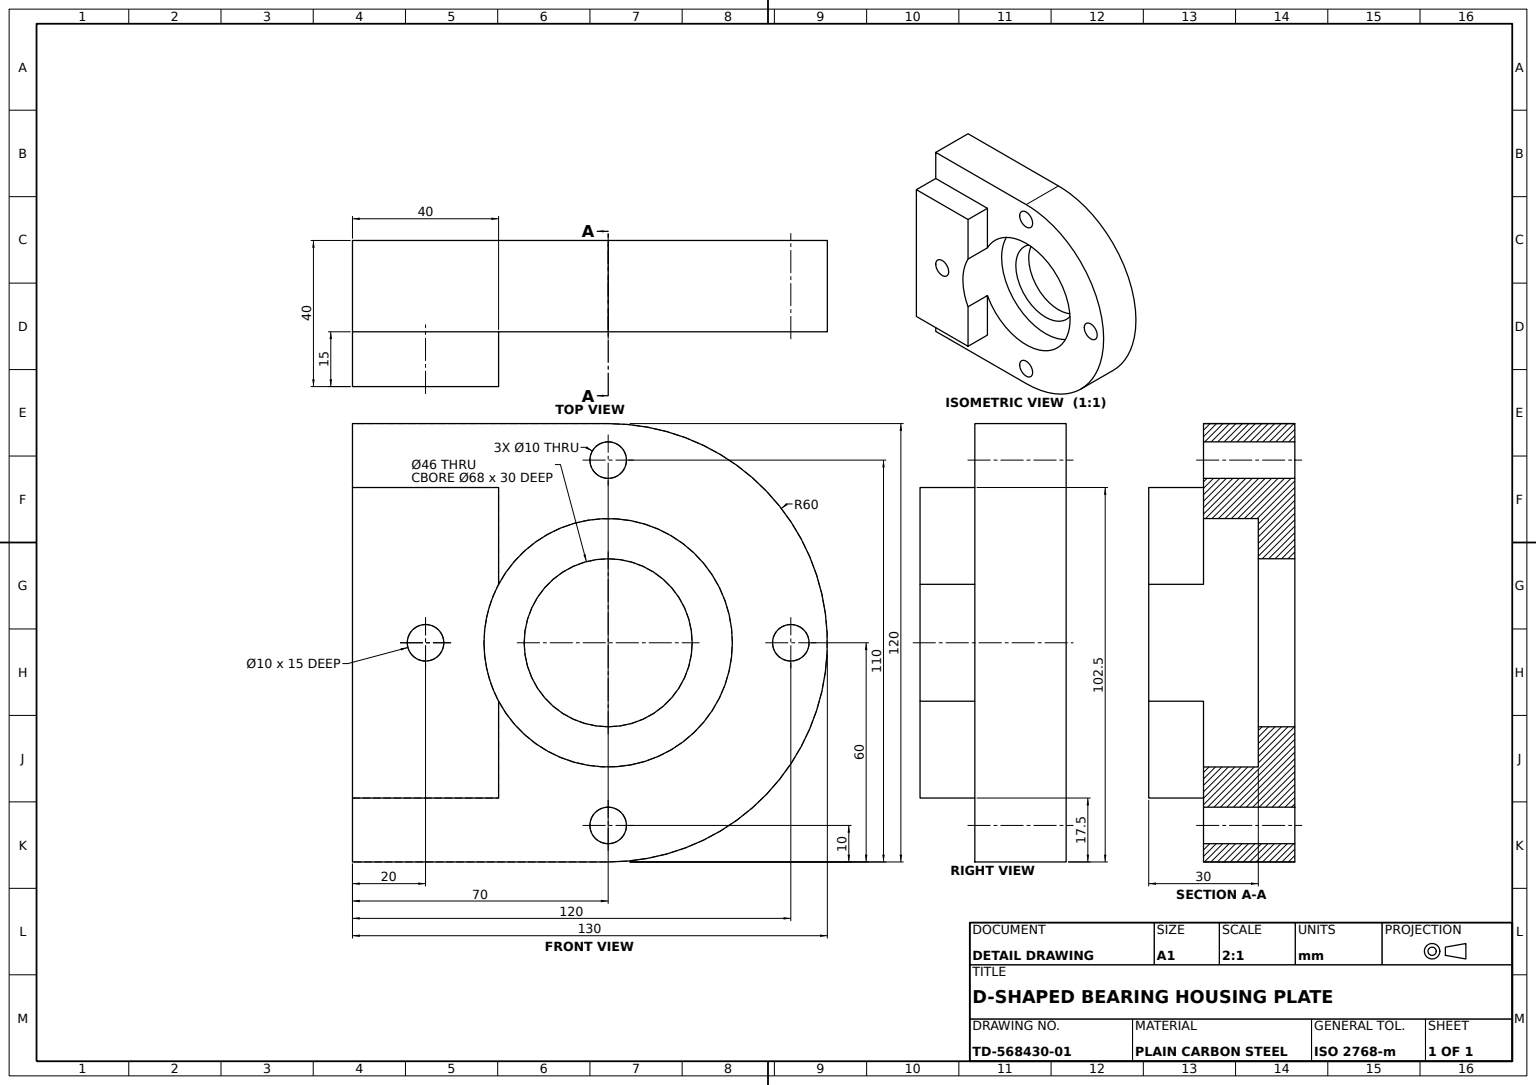
from build123d import *
from build123d.topology import SkipClean

# Parameters (mm, degrees)
BASE_PLATE_DEPTH           = 25
SIDE_BLOCK_SKETCH_W        = 40
SIDE_BLOCK_SKETCH_H        = 85
SIDE_BLOCK_DEPTH           = 15
COUNTERBORE_68_SKETCH_R    = 34
COUNTERBORE_68_DEPTH       = 15
BLOCK_RELIEF_68_DEPTH      = 15
BORE_46_SKETCH_R           = 23
BORE_46_DEPTH              = 15
BLOCK_HOLE_10_SKETCH_R     = 5
BLOCK_HOLE_10_DEPTH        = 15
MOUNTING_HOLES_SKETCH_R    = 5
MOUNTING_HOLES_3X_10_DEPTH = 25


with BuildPart() as part:
    # Base Plate Sketch → Base Plate (new body)
    with BuildSketch(Plane.XY):
        with BuildLine():
            Line((0, 0), (70, 0))
            ThreePointArc((70, 0), (130, 60), (70, 120))
            Line((70, 120), (0, 120))
            Line((0, 120), (0, 0))
        make_face()
    extrude(amount=BASE_PLATE_DEPTH)

    # Side Block Sketch → Side Block (add)
    with BuildSketch(Plane.XY.offset(25)):
        with Locations((20, 60)):
            Rectangle(SIDE_BLOCK_SKETCH_W, SIDE_BLOCK_SKETCH_H)
    extrude(amount=SIDE_BLOCK_DEPTH)

    # Counterbore Ø68 Sketch → Counterbore Ø68 (cut)
    with BuildSketch(Plane.XY.offset(25)):
        with Locations((70, 60)):
            Circle(COUNTERBORE_68_SKETCH_R)
    extrude(amount=-COUNTERBORE_68_DEPTH, mode=Mode.SUBTRACT)

    # Block Relief Ø68 Sketch → Block Relief Ø68 (cut)
    with SkipClean():  # the faces are left unmerged after this step: merging them gives an invalid solid
        with BuildSketch(Plane.XY.offset(40)):
            with BuildLine():
                Line((40, 76), (40, 44))
                ThreePointArc((40, 44), (36, 60), (40, 76))
            make_face()
        extrude(amount=-BLOCK_RELIEF_68_DEPTH, mode=Mode.SUBTRACT)

    # Bore Ø46 Sketch → Bore Ø46 (cut)
    with SkipClean():  # the faces are left unmerged after this step: merging them gives an invalid solid
        with BuildSketch(Plane.XY.offset(10)):
            with Locations((70, 60)):
                Circle(BORE_46_SKETCH_R)
        extrude(amount=-BORE_46_DEPTH, mode=Mode.SUBTRACT)

    # Block Hole Ø10 Sketch → Block Hole Ø10 (cut)
    with SkipClean():  # the faces are left unmerged after this step: merging them gives an invalid solid
        with BuildSketch(Plane.XY.offset(40)):
            with Locations((20, 60)):
                Circle(BLOCK_HOLE_10_SKETCH_R)
        extrude(amount=-BLOCK_HOLE_10_DEPTH, mode=Mode.SUBTRACT)

    # Mounting Holes Sketch → Mounting Holes 3xØ10 (cut)
    with SkipClean():  # the faces are left unmerged after this step: merging them gives an invalid solid
        with BuildSketch(Plane.XY.offset(25)):
            with Locations((70, 110)):
                Circle(MOUNTING_HOLES_SKETCH_R)
            with Locations((120, 60)):
                Circle(MOUNTING_HOLES_SKETCH_R)
            with Locations((70, 10)):
                Circle(MOUNTING_HOLES_SKETCH_R)
        extrude(amount=-MOUNTING_HOLES_3X_10_DEPTH, mode=Mode.SUBTRACT)


solid = part.part
